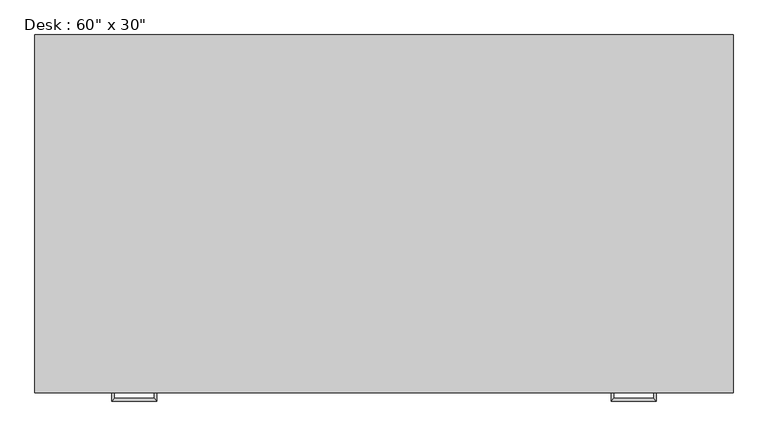
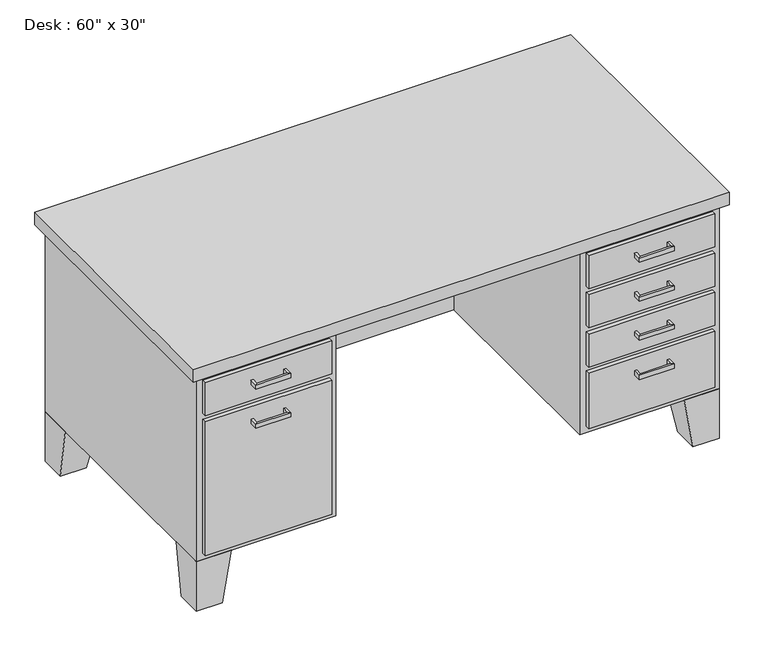
"""IFC4 building model written with IfcOpenShell, lengths in millimetres: furniture geometry."""

from ifc_helpers import new_model, si_unit, frame, origin, place, context, project, spatial, polyline, outline, extrude, faceted_brep, source, transform, mapped, element, save


def furniture_013ab306(model_context):
    return source(origin(), model_context, "Body", "SolidModel", [
        extrude(outline(polyline([(19.05, 0.0), (387.35, 0.0), (387.35, -12.7), (19.05, -12.7), (19.05, 0.0)])), frame((0.0, 0.0, 603.25), z_axis=(0.0, 0.0, 1.0), x_axis=(1.0, 0.0, 0.0)), (0.0, 0.0, 1.0), 101.6),
        extrude(outline(polyline([(19.05, 0.0), (387.35, 0.0), (387.35, -12.7), (19.05, -12.7), (19.05, 0.0)])), frame((0.0, 0.0, 171.45), z_axis=(0.0, 0.0, 1.0), x_axis=(1.0, 0.0, 0.0)), (0.0, 0.0, 1.0), 412.75),
        extrude(outline(polyline([(1136.65, 0.0), (1504.95, 0.0), (1504.95, -12.7), (1136.65, -12.7), (1136.65, 0.0)])), frame((0.0, 0.0, 603.25), z_axis=(0.0, 0.0, 1.0), x_axis=(1.0, 0.0, 0.0)), (0.0, 0.0, 1.0), 101.6),
        extrude(outline(polyline([(1136.65, 0.0), (1504.95, 0.0), (1504.95, -12.7), (1136.65, -12.7), (1136.65, 0.0)])), frame((0.0, 0.0, 171.45), z_axis=(0.0, 0.0, 1.0), x_axis=(1.0, 0.0, 0.0)), (0.0, 0.0, 1.0), 171.45),
        extrude(outline(polyline([(1136.65, 0.0), (1504.95, 0.0), (1504.95, -12.7), (1136.65, -12.7), (1136.65, 0.0)])), frame((0.0, 0.0, 482.6), z_axis=(0.0, 0.0, 1.0), x_axis=(1.0, 0.0, 0.0)), (0.0, 0.0, 1.0), 101.6),
        extrude(outline(polyline([(1136.65, 0.0), (1504.95, 0.0), (1504.95, -12.7), (1136.65, -12.7), (1136.65, 0.0)])), frame((0.0, 0.0, 361.95), z_axis=(0.0, 0.0, 1.0), x_axis=(1.0, 0.0, 0.0)), (0.0, 0.0, 1.0), 101.6),
        faceted_brep([(101.6, 0.0, 152.4), (101.6, 101.6, 152.4), (0.0, 101.6, 152.4), (0.0, 0.0, 152.4), (76.2, 0.0, 0.0), (0.0, 0.0, 0.0), (0.0, 76.2, 0.0), (76.2, 76.2, 0.0)], [[[0, 1, 2, 3]], [[4, 5, 6, 7]], [[4, 7, 1, 0]], [[7, 6, 2, 1]], [[6, 5, 3, 2]], [[5, 4, 0, 3]]]),
        faceted_brep([(101.6, 762.0, 152.4), (0.0, 762.0, 152.4), (0.0, 660.4, 152.4), (101.6, 660.4, 152.4), (76.2, 762.0, 0.0), (76.2, 685.8, 0.0), (0.0, 685.8, 0.0), (0.0, 762.0, 0.0)], [[[0, 1, 2, 3]], [[4, 5, 6, 7]], [[4, 7, 1, 0]], [[7, 6, 2, 1]], [[6, 5, 3, 2]], [[5, 4, 0, 3]]]),
        faceted_brep([(1422.4, 762.0, 152.4), (1422.4, 660.4, 152.4), (1524.0, 660.4, 152.4), (1524.0, 762.0, 152.4), (1447.8, 762.0, 0.0), (1524.0, 762.0, 0.0), (1524.0, 685.8, 0.0), (1447.8, 685.8, 0.0)], [[[0, 1, 2, 3]], [[4, 5, 6, 7]], [[4, 7, 1, 0]], [[7, 6, 2, 1]], [[6, 5, 3, 2]], [[5, 4, 0, 3]]]),
        faceted_brep([(1422.4, 0.0, 152.4), (1524.0, 0.0, 152.4), (1524.0, 101.6, 152.4), (1422.4, 101.6, 152.4), (1447.8, 0.0, 0.0), (1447.8, 76.2, 0.0), (1524.0, 76.2, 0.0), (1524.0, 0.0, 0.0)], [[[0, 1, 2, 3]], [[4, 5, 6, 7]], [[4, 7, 1, 0]], [[7, 6, 2, 1]], [[6, 5, 3, 2]], [[5, 4, 0, 3]]]),
        extrude(outline(polyline([(-19.05, -19.05), (-19.05, 781.05), (1543.05, 781.05), (1543.05, -19.05), (-19.05, -19.05)])), frame((0.0, 0.0, 723.9), z_axis=(0.0, 0.0, 1.0), x_axis=(1.0, 0.0, 0.0)), (0.0, 0.0, 1.0), 38.1),
        extrude(outline(polyline([(1117.6, 0.0), (1117.6, 635.0), (406.4, 635.0), (406.4, 0.0), (0.0, 0.0), (0.0, 762.0), (1524.0, 762.0), (1524.0, 0.0), (1117.6, 0.0)])), frame((0.0, 0.0, 152.4), z_axis=(0.0, 0.0, 1.0), x_axis=(1.0, 0.0, 0.0)), (0.0, 0.0, 1.0), 571.5),
        faceted_brep([(158.75, -12.7, 546.1), (158.75, -12.7, 533.4), (152.4, -12.7, 533.4), (152.4, -12.7, 546.1), (158.75, -31.75, 546.1), (158.75, -31.75, 533.4), (152.4, -38.1, 533.4), (152.4, -38.1, 546.1), (247.65, -31.75, 546.1), (247.65, -31.75, 533.4), (254.0, -38.1, 533.4), (254.0, -38.1, 546.1), (247.65, -12.7, 546.1), (254.0, -12.7, 546.1), (254.0, -12.7, 533.4), (247.65, -12.7, 533.4)], [[[0, 1, 2, 3]], [[1, 0, 4, 5]], [[2, 1, 5, 6]], [[3, 2, 6, 7]], [[0, 3, 7, 4]], [[5, 4, 8, 9]], [[6, 5, 9, 10]], [[7, 6, 10, 11]], [[4, 7, 11, 8]], [[12, 13, 14, 15]], [[9, 8, 12, 15]], [[10, 9, 15, 14]], [[11, 10, 14, 13]], [[8, 11, 13, 12]]]),
        faceted_brep([(158.75, -12.7, 666.75), (158.75, -12.7, 654.05), (152.4, -12.7, 654.05), (152.4, -12.7, 666.75), (158.75, -31.75, 666.75), (158.75, -31.75, 654.05), (152.4, -38.1, 654.05), (152.4, -38.1, 666.75), (247.65, -31.75, 666.75), (247.65, -31.75, 654.05), (254.0, -38.1, 654.05), (254.0, -38.1, 666.75), (247.65, -12.7, 666.75), (254.0, -12.7, 666.75), (254.0, -12.7, 654.05), (247.65, -12.7, 654.05)], [[[0, 1, 2, 3]], [[1, 0, 4, 5]], [[2, 1, 5, 6]], [[3, 2, 6, 7]], [[0, 3, 7, 4]], [[5, 4, 8, 9]], [[6, 5, 9, 10]], [[7, 6, 10, 11]], [[4, 7, 11, 8]], [[12, 13, 14, 15]], [[9, 8, 12, 15]], [[10, 9, 15, 14]], [[11, 10, 14, 13]], [[8, 11, 13, 12]]]),
        faceted_brep([(1365.25, -12.7, 304.8), (1371.6, -12.7, 304.8), (1371.6, -12.7, 292.1), (1365.25, -12.7, 292.1), (1365.25, -31.75, 304.8), (1371.6, -38.1, 304.8), (1371.6, -38.1, 292.1), (1365.25, -31.75, 292.1), (1276.35, -31.75, 304.8), (1270.0, -38.1, 304.8), (1270.0, -38.1, 292.1), (1276.35, -31.75, 292.1), (1276.35, -12.7, 304.8), (1276.35, -12.7, 292.1), (1270.0, -12.7, 292.1), (1270.0, -12.7, 304.8)], [[[0, 1, 2, 3]], [[1, 0, 4, 5]], [[2, 1, 5, 6]], [[3, 2, 6, 7]], [[0, 3, 7, 4]], [[5, 4, 8, 9]], [[6, 5, 9, 10]], [[7, 6, 10, 11]], [[4, 7, 11, 8]], [[12, 13, 14, 15]], [[9, 8, 12, 15]], [[10, 9, 15, 14]], [[11, 10, 14, 13]], [[8, 11, 13, 12]]]),
        faceted_brep([(1365.25, -12.7, 425.45), (1371.6, -12.7, 425.45), (1371.6, -12.7, 412.75), (1365.25, -12.7, 412.75), (1365.25, -31.75, 425.45), (1371.6, -38.1, 425.45), (1371.6, -38.1, 412.75), (1365.25, -31.75, 412.75), (1276.35, -31.75, 425.45), (1270.0, -38.1, 425.45), (1270.0, -38.1, 412.75), (1276.35, -31.75, 412.75), (1276.35, -12.7, 425.45), (1276.35, -12.7, 412.75), (1270.0, -12.7, 412.75), (1270.0, -12.7, 425.45)], [[[0, 1, 2, 3]], [[1, 0, 4, 5]], [[2, 1, 5, 6]], [[3, 2, 6, 7]], [[0, 3, 7, 4]], [[5, 4, 8, 9]], [[6, 5, 9, 10]], [[7, 6, 10, 11]], [[4, 7, 11, 8]], [[12, 13, 14, 15]], [[9, 8, 12, 15]], [[10, 9, 15, 14]], [[11, 10, 14, 13]], [[8, 11, 13, 12]]]),
        faceted_brep([(1365.25, -12.7, 546.1), (1371.6, -12.7, 546.1), (1371.6, -12.7, 533.4), (1365.25, -12.7, 533.4), (1365.25, -31.75, 546.1), (1371.6, -38.1, 546.1), (1371.6, -38.1, 533.4), (1365.25, -31.75, 533.4), (1276.35, -31.75, 546.1), (1270.0, -38.1, 546.1), (1270.0, -38.1, 533.4), (1276.35, -31.75, 533.4), (1276.35, -12.7, 546.1), (1276.35, -12.7, 533.4), (1270.0, -12.7, 533.4), (1270.0, -12.7, 546.1)], [[[0, 1, 2, 3]], [[1, 0, 4, 5]], [[2, 1, 5, 6]], [[3, 2, 6, 7]], [[0, 3, 7, 4]], [[5, 4, 8, 9]], [[6, 5, 9, 10]], [[7, 6, 10, 11]], [[4, 7, 11, 8]], [[12, 13, 14, 15]], [[9, 8, 12, 15]], [[10, 9, 15, 14]], [[11, 10, 14, 13]], [[8, 11, 13, 12]]]),
        faceted_brep([(1365.25, -12.7, 666.75), (1371.6, -12.7, 666.75), (1371.6, -12.7, 654.05), (1365.25, -12.7, 654.05), (1365.25, -31.75, 666.75), (1371.6, -38.1, 666.75), (1371.6, -38.1, 654.05), (1365.25, -31.75, 654.05), (1276.35, -31.75, 666.75), (1270.0, -38.1, 666.75), (1270.0, -38.1, 654.05), (1276.35, -31.75, 654.05), (1276.35, -12.7, 666.75), (1276.35, -12.7, 654.05), (1270.0, -12.7, 654.05), (1270.0, -12.7, 666.75)], [[[0, 1, 2, 3]], [[1, 0, 4, 5]], [[2, 1, 5, 6]], [[3, 2, 6, 7]], [[0, 3, 7, 4]], [[5, 4, 8, 9]], [[6, 5, 9, 10]], [[7, 6, 10, 11]], [[4, 7, 11, 8]], [[12, 13, 14, 15]], [[9, 8, 12, 15]], [[10, 9, 15, 14]], [[11, 10, 14, 13]], [[8, 11, 13, 12]]]),
    ])


if __name__ == "__main__":
    model = new_model("IFC4")
    model_context = context("Model", 3, world=origin())
    ifc_project = project(units=[si_unit("LENGTHUNIT", "METRE", prefix="MILLI")], contexts=[model_context])
    site = spatial("IfcSite", under=ifc_project)
    building = spatial("IfcBuilding", under=site)
    placement = place(None, origin())
    furniture_shape = furniture_013ab306(model_context)
    element("IfcFurniture", 1, ObjectType="Desk : 60\" x 30\"", at=placement, inside=building, context=model_context, shape_type="MappedRepresentation", body=[
        mapped(furniture_shape, transform((0.0, 0.0, 0.0), x_axis=(1.0, 0.0, 0.0), y_axis=(0.0, 1.0, 0.0), z_axis=(0.0, 0.0, 1.0))),
    ])
    save(model, "model.ifc")

# Revit data of these elements
# Type "Desk : 60\" x 30\""
#   Assembly Code = "E2020200"
#   Depth = 2' - 6"
#   Height = 2' - 6"
#   Leg Height = 0' - 6"
#   Width = 5' - 0"
#   Body Material = Laminate, Ivory, Matte
#   Handle/Leg Material = Steel, Chrome Plated
#   Top Material = Cherry
#   Default Elevation = 0
# Element 1 (IfcFurniture, "Desk : 60\" x 30\"")
#   Materials on its faces: "Steel, Chrome Plated", "Laminate, Ivory, Matte", "Cherry"
# Materials
#   "Laminate, Ivory, Matte": class "Plastic", colour RGB 247 247 239, transparency 0, Description = "Plastic Laminate - Ivory, Matte", Cost = 0
#   "Steel, Chrome Plated": class "Metal", colour RGB 17 17 17, transparency 0, Description = "Chromiuim plated steel", Cost = 0
#   "Cherry": class "Wood", colour RGB 226 177 128, transparency 0, Description = "Prunus Serotina", Cost = 0
